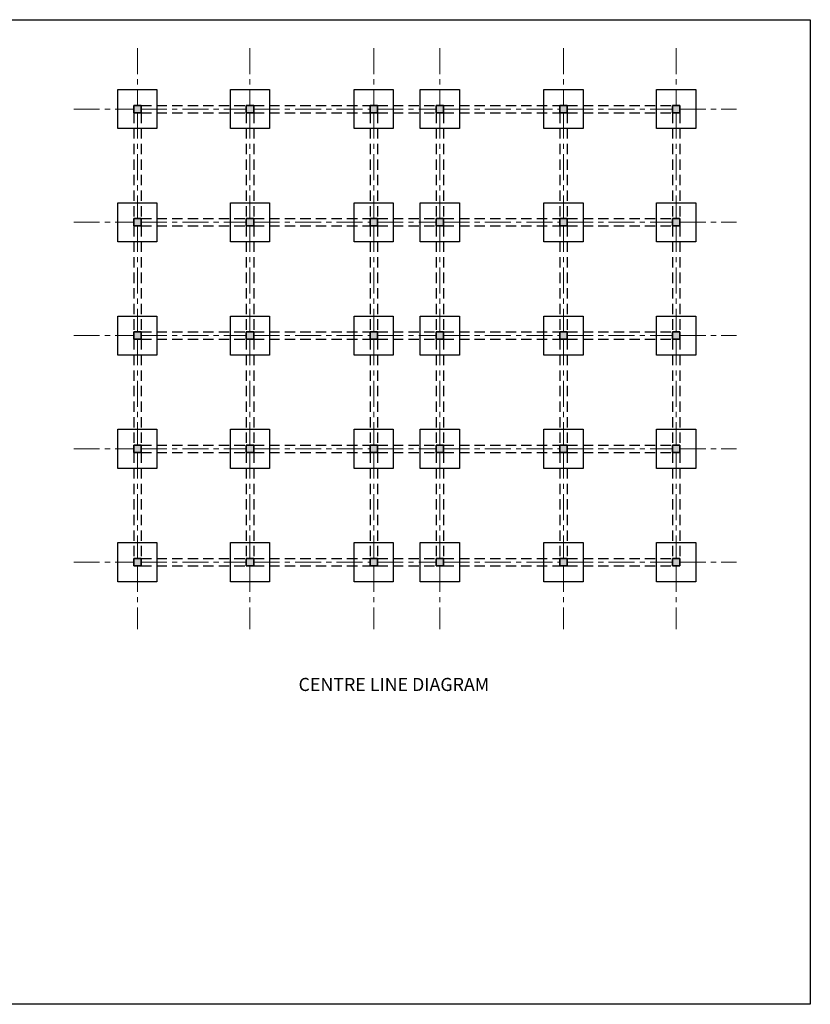
# Model space of a CAD drawing. Units: inches. Extents: x 9239 to 26065, y 6728 to 14611.
# Tile 4 of 12: x 10240 to 11208, y 6728 to 7934. Entities that reach past the tile are written whole.
import ezdxf

# ---------------------------------------------------------------- set-up
doc = ezdxf.new("R2010")
doc.units = ezdxf.units.IN
doc.header["$MEASUREMENT"] = 0
doc.linetypes.add('CENTER', pattern=[50.8, 31.75, -6.35, 6.35, -6.35])
doc.linetypes.add('DASHED', pattern=[19.05, 12.7, -6.35])
for name, color, linetype, lineweight in [('A-ANNO-TEXT', 7, 'Continuous', 18), ('A-FLOR-STRS', 3, 'Continuous', 25), ('A-GRID', 3, 'CENTER', 18), ('S-BEAM', 4, 'DASHED', 25), ('S-COLS', 1, 'Continuous', 35), ('S-FNDN', 6, 'Continuous', 25), ('S-PATT', 252, 'Continuous', 13)]:
    doc.layers.add(name, color=color, linetype=linetype, lineweight=lineweight)
doc.styles.get("Standard").update_dxf_attribs({"font": 'arial.ttf'})

msp = doc.modelspace()

# ---------------------------------------------------------------- hatches: boundary and pattern name
at = {"layer": 'S-PATT'}
h = msp.add_hatch(color=256, dxfattribs=at)
h.dxf.hatch_style = 1
h.paths.add_polyline_path([(10388.37, 7820.07), (10388.37, 7829.07), (10379.37, 7829.07), (10379.37, 7820.07)])
h.paths.add_polyline_path([(10517.37, 7829.07), (10517.37, 7820.07), (10526.37, 7820.07), (10526.37, 7829.07)])
h.paths.add_polyline_path([(10668.87, 7820.07), (10677.87, 7820.07), (10677.87, 7829.07), (10668.87, 7829.07)])
h.paths.add_polyline_path([(10758.87, 7820.07), (10758.87, 7829.07), (10749.87, 7829.07), (10749.87, 7820.07)])
h.paths.add_polyline_path([(10910.37, 7829.07), (10901.37, 7829.07), (10901.37, 7820.07), (10910.37, 7820.07)])
h.paths.add_polyline_path([(11048.37, 7829.07), (11039.37, 7829.07), (11039.37, 7820.07), (11048.37, 7820.07)])
h.paths.add_polyline_path([(10379.37, 7681.32), (10388.37, 7681.32), (10388.37, 7690.32), (10379.37, 7690.32)])
h.paths.add_polyline_path([(10526.37, 7681.32), (10526.37, 7690.32), (10517.37, 7690.32), (10517.37, 7681.32)])
h.paths.add_polyline_path([(10668.87, 7681.32), (10677.87, 7681.32), (10677.87, 7690.32), (10668.87, 7690.32)])
h.paths.add_polyline_path([(10758.87, 7681.32), (10758.87, 7690.32), (10749.87, 7690.32), (10749.87, 7681.32)])
h.paths.add_polyline_path([(10910.37, 7690.32), (10901.37, 7690.32), (10901.37, 7681.32), (10910.37, 7681.32)])
h.paths.add_polyline_path([(11039.37, 7690.32), (11039.37, 7681.32), (11048.37, 7681.32), (11048.37, 7690.32)])
h.paths.add_polyline_path([(10388.37, 7551.57), (10379.37, 7551.57), (10379.37, 7542.57), (10388.37, 7542.57)])
h.paths.add_polyline_path([(10526.37, 7542.57), (10526.37, 7551.57), (10517.37, 7551.57), (10517.37, 7542.57)])
h.paths.add_polyline_path([(10677.87, 7551.57), (10668.87, 7551.57), (10668.87, 7542.57), (10677.87, 7542.57)])
h.paths.add_polyline_path([(10749.87, 7542.57), (10758.87, 7542.57), (10758.87, 7551.57), (10749.87, 7551.57)])
h.paths.add_polyline_path([(10910.37, 7551.57), (10901.37, 7551.57), (10901.37, 7542.57), (10910.37, 7542.57)])
h.paths.add_polyline_path([(11048.37, 7542.57), (11048.37, 7551.57), (11039.37, 7551.57), (11039.37, 7542.57)])
h.paths.add_polyline_path([(10388.37, 7403.82), (10388.37, 7412.82), (10379.37, 7412.82), (10379.37, 7403.82)])
h.paths.add_polyline_path([(10517.37, 7403.82), (10526.37, 7403.82), (10526.37, 7412.82), (10517.37, 7412.82)])
h.paths.add_polyline_path([(10668.87, 7403.82), (10677.87, 7403.82), (10677.87, 7412.82), (10668.87, 7412.82)])
h.paths.add_polyline_path([(10749.87, 7403.82), (10758.87, 7403.82), (10758.87, 7412.82), (10749.87, 7412.82)])
h.paths.add_polyline_path([(10910.37, 7412.82), (10901.37, 7412.82), (10901.37, 7403.82), (10910.37, 7403.82)])
h.paths.add_polyline_path([(11048.37, 7403.82), (11048.37, 7412.82), (11039.37, 7412.82), (11039.37, 7403.82)])
h.paths.add_polyline_path([(11048.37, 7265.07), (11048.37, 7274.07), (11039.37, 7274.07), (11039.37, 7265.07)])
h.paths.add_polyline_path([(10901.37, 7265.07), (10910.37, 7265.07), (10910.37, 7274.07), (10901.37, 7274.07)])
h.paths.add_polyline_path([(10758.87, 7265.07), (10758.87, 7274.07), (10749.87, 7274.07), (10749.87, 7265.07)])
h.paths.add_polyline_path([(10668.87, 7265.07), (10677.87, 7265.07), (10677.87, 7274.07), (10668.87, 7274.07)])
h.paths.add_polyline_path([(10517.37, 7265.07), (10526.37, 7265.07), (10526.37, 7274.07), (10517.37, 7274.07)])
h.paths.add_polyline_path([(10379.37, 7274.07), (10379.37, 7265.07), (10388.37, 7265.07), (10388.37, 7274.07)])

# ---------------------------------------------------------------- linework, layer by layer
at = {"layer": 'A-FLOR-STRS'}
msp.add_lwpolyline([(9238.6, 7933.95), (11208.24, 7933.95), (11208.24, 6728.19), (9238.6, 6728.19)], close=True, dxfattribs=at)
at = {"layer": 'A-GRID'}
for p, q in [((10383.87, 7899.11), (10383.87, 7829.07)), ((10521.87, 7899.11), (10521.87, 7829.07)), ((10673.37, 7899.11), (10673.37, 7829.07)), ((10754.37, 7899.11), (10754.37, 7829.07)), ((10905.87, 7899.11), (10905.87, 7829.07)), ((11043.87, 7899.11), (11043.87, 7829.07)), ((10305.95, 7824.57), (10379.37, 7824.57)), ((10383.87, 7820.07), (10383.87, 7800.57)), ((10383.87, 7820.07), (10383.87, 7690.32)), ((10388.37, 7824.57), (10517.37, 7824.57)), ((10521.87, 7820.07), (10521.87, 7690.32)), ((10526.37, 7824.57), (10668.87, 7824.57)), ((10673.37, 7820.07), (10673.37, 7690.32)), ((10677.87, 7824.57), (10749.87, 7824.57)), ((10754.37, 7820.07), (10754.37, 7690.32)), ((10758.87, 7824.57), (10901.37, 7824.57)), ((10905.87, 7820.07), (10905.87, 7690.32)), ((10910.37, 7824.57), (11039.37, 7824.57)), ((11043.87, 7820.07), (11043.87, 7690.32)), ((11048.37, 7824.57), (11117.64, 7824.57)), ((10305.95, 7685.82), (10379.37, 7685.82)), ((10383.87, 7681.32), (10383.87, 7551.57)), ((10388.37, 7685.82), (10517.37, 7685.82)), ((10521.87, 7681.32), (10521.87, 7551.57)), ((10526.37, 7685.82), (10668.87, 7685.82)), ((10673.37, 7681.32), (10673.37, 7551.57)), ((10677.87, 7685.82), (10749.87, 7685.82)), ((10754.37, 7681.32), (10754.37, 7551.57)), ((10758.87, 7685.82), (10901.37, 7685.82)), ((10905.87, 7681.32), (10905.87, 7551.57)), ((10910.37, 7685.82), (11039.37, 7685.82)), ((11043.87, 7681.32), (11043.87, 7551.57)), ((11048.37, 7685.82), (11117.64, 7685.82)), ((10305.95, 7547.07), (10379.37, 7547.07)), ((10383.87, 7542.57), (10383.87, 7412.82)), ((10388.37, 7547.07), (10517.37, 7547.07)), ((10521.87, 7542.57), (10521.87, 7412.82)), ((10526.37, 7547.07), (10668.87, 7547.07)), ((10673.37, 7542.57), (10673.37, 7412.82)), ((10677.87, 7547.07), (10749.87, 7547.07)), ((10754.37, 7542.57), (10754.37, 7412.82)), ((10758.87, 7547.07), (10901.37, 7547.07)), ((10905.87, 7542.57), (10905.87, 7412.82)), ((10910.37, 7547.07), (11039.37, 7547.07)), ((11043.87, 7542.57), (11043.87, 7412.82)), ((11048.37, 7547.07), (11117.64, 7547.07)), ((10305.95, 7408.32), (10379.37, 7408.32)), ((10383.87, 7403.82), (10383.87, 7274.07)), ((10388.37, 7408.32), (10517.37, 7408.32)), ((10521.87, 7403.82), (10521.87, 7274.07)), ((10526.37, 7408.32), (10668.87, 7408.32)), ((10673.37, 7403.82), (10673.37, 7274.07)), ((10677.87, 7408.32), (10749.87, 7408.32)), ((10754.37, 7403.82), (10754.37, 7274.07)), ((10758.87, 7408.32), (10901.37, 7408.32)), ((10905.87, 7403.82), (10905.87, 7274.07)), ((10910.37, 7408.32), (11039.37, 7408.32)), ((11043.87, 7403.82), (11043.87, 7274.07)), ((11048.37, 7408.32), (11117.64, 7408.32)), ((10305.95, 7269.57), (10379.37, 7269.57)), ((10383.87, 7265.07), (10383.87, 7187.6)), ((10388.37, 7269.57), (10517.37, 7269.57)), ((10521.87, 7265.07), (10521.87, 7187.6)), ((10526.37, 7269.57), (10668.87, 7269.57)), ((10673.37, 7265.07), (10673.37, 7187.6)), ((10677.87, 7269.57), (10749.87, 7269.57)), ((10677.87, 7269.57), (10749.87, 7269.57)), ((10754.37, 7265.07), (10754.37, 7187.6)), ((10758.87, 7269.57), (10901.37, 7269.57)), ((10905.87, 7265.07), (10905.87, 7187.6)), ((10910.37, 7269.57), (11039.37, 7269.57)), ((11043.87, 7265.07), (11043.87, 7187.6)), ((11048.37, 7269.57), (11117.64, 7269.57))]:
    msp.add_line(p, q, dxfattribs=at)
at = {"layer": 'S-BEAM'}
for p, q in [((10388.37, 7829.07), (10517.37, 7829.07)), ((10526.37, 7829.07), (10668.87, 7829.07)), ((10677.87, 7829.07), (10749.87, 7829.07)), ((10758.87, 7829.07), (10901.37, 7829.07)), ((10910.37, 7829.07), (11039.37, 7829.07)), ((10379.37, 7820.07), (10379.37, 7690.32)), ((10388.37, 7820.07), (10388.37, 7690.32)), ((10388.37, 7820.07), (10517.37, 7820.07)), ((10517.37, 7820.07), (10517.37, 7690.32)), ((10526.37, 7820.07), (10526.37, 7690.32)), ((10526.37, 7820.07), (10668.87, 7820.07)), ((10668.87, 7820.07), (10668.87, 7690.32)), ((10677.87, 7820.07), (10677.87, 7690.32)), ((10677.87, 7820.07), (10749.87, 7820.07)), ((10749.87, 7820.07), (10749.87, 7690.32)), ((10758.87, 7820.07), (10758.87, 7690.32)), ((10758.87, 7820.07), (10901.37, 7820.07)), ((10901.37, 7820.07), (10901.37, 7690.32)), ((10910.37, 7820.07), (10910.37, 7690.32)), ((10910.37, 7820.07), (11039.37, 7820.07)), ((11039.37, 7820.07), (11039.37, 7690.32)), ((11048.37, 7820.07), (11048.37, 7690.32)), ((10379.37, 7681.32), (10379.37, 7551.57)), ((10388.37, 7690.32), (10517.37, 7690.32)), ((10388.37, 7681.32), (10388.37, 7551.57)), ((10388.37, 7681.32), (10517.37, 7681.32)), ((10517.37, 7681.32), (10517.37, 7551.57)), ((10526.37, 7690.32), (10668.87, 7690.32)), ((10526.37, 7681.32), (10526.37, 7551.57)), ((10526.37, 7681.32), (10668.87, 7681.32)), ((10668.87, 7681.32), (10668.87, 7551.57)), ((10677.87, 7690.32), (10749.87, 7690.32)), ((10677.87, 7681.32), (10677.87, 7551.57)), ((10677.87, 7681.32), (10749.87, 7681.32)), ((10749.87, 7681.32), (10749.87, 7551.57)), ((10758.87, 7690.32), (10901.37, 7690.32)), ((10758.87, 7681.32), (10758.87, 7551.57)), ((10758.87, 7681.32), (10901.37, 7681.32)), ((10901.37, 7681.32), (10901.37, 7551.57)), ((10910.37, 7690.32), (11039.37, 7690.32)), ((10910.37, 7681.32), (10910.37, 7551.57)), ((10910.37, 7681.32), (11039.37, 7681.32)), ((11039.37, 7681.32), (11039.37, 7551.57)), ((11048.37, 7681.32), (11048.37, 7551.57)), ((10388.37, 7551.57), (10517.37, 7551.57)), ((10526.37, 7551.57), (10668.87, 7551.57)), ((10677.87, 7551.57), (10749.87, 7551.57)), ((10758.87, 7551.57), (10901.37, 7551.57)), ((10910.37, 7551.57), (11039.37, 7551.57)), ((10379.37, 7542.57), (10379.37, 7412.82)), ((10388.37, 7542.57), (10388.37, 7412.82)), ((10388.37, 7542.57), (10517.37, 7542.57)), ((10517.37, 7542.57), (10517.37, 7412.82)), ((10526.37, 7542.57), (10526.37, 7412.82)), ((10526.37, 7542.57), (10668.87, 7542.57)), ((10668.87, 7542.57), (10668.87, 7412.82)), ((10677.87, 7542.57), (10677.87, 7412.82)), ((10677.87, 7542.57), (10749.87, 7542.57)), ((10749.87, 7542.57), (10749.87, 7412.82)), ((10758.87, 7542.57), (10758.87, 7412.82)), ((10758.87, 7542.57), (10901.37, 7542.57)), ((10901.37, 7542.57), (10901.37, 7412.82)), ((10910.37, 7542.57), (10910.37, 7412.82)), ((10910.37, 7542.57), (11039.37, 7542.57)), ((11039.37, 7542.57), (11039.37, 7412.82)), ((11048.37, 7542.57), (11048.37, 7412.82)), ((10379.37, 7403.82), (10379.37, 7274.07)), ((10388.37, 7412.82), (10517.37, 7412.82)), ((10388.37, 7403.82), (10388.37, 7274.07)), ((10388.37, 7403.82), (10517.37, 7403.82)), ((10517.37, 7403.82), (10517.37, 7274.07)), ((10526.37, 7412.82), (10668.87, 7412.82)), ((10526.37, 7403.82), (10526.37, 7274.07)), ((10526.37, 7403.82), (10668.87, 7403.82)), ((10668.87, 7403.82), (10668.87, 7274.07)), ((10677.87, 7412.82), (10749.87, 7412.82)), ((10677.87, 7403.82), (10677.87, 7274.07)), ((10677.87, 7403.82), (10749.87, 7403.82)), ((10749.87, 7403.82), (10749.87, 7274.07)), ((10758.87, 7412.82), (10901.37, 7412.82)), ((10758.87, 7403.82), (10758.87, 7274.07)), ((10758.87, 7403.82), (10901.37, 7403.82)), ((10901.37, 7403.82), (10901.37, 7274.07)), ((10910.37, 7412.82), (11039.37, 7412.82)), ((10910.37, 7403.82), (10910.37, 7274.07)), ((10910.37, 7403.82), (11039.37, 7403.82)), ((11039.37, 7403.82), (11039.37, 7274.07)), ((11048.37, 7403.82), (11048.37, 7274.07)), ((10388.37, 7274.07), (10517.37, 7274.07)), ((10526.37, 7274.07), (10668.87, 7274.07)), ((10677.87, 7274.07), (10749.87, 7274.07)), ((10758.87, 7274.07), (10901.37, 7274.07)), ((10910.37, 7274.07), (11039.37, 7274.07)), ((10388.37, 7265.07), (10517.37, 7265.07)), ((10526.37, 7265.07), (10668.87, 7265.07)), ((10677.87, 7265.07), (10749.87, 7265.07)), ((10758.87, 7265.07), (10901.37, 7265.07)), ((10910.37, 7265.07), (11039.37, 7265.07))]:
    msp.add_line(p, q, dxfattribs=at)
at = {"layer": 'S-COLS'}
for p, q in [((10379.37, 7829.07), (10388.37, 7829.07)), ((10379.37, 7820.07), (10379.37, 7829.07)), ((10388.37, 7829.07), (10388.37, 7820.07)), ((10517.37, 7829.07), (10526.37, 7829.07)), ((10517.37, 7820.07), (10517.37, 7829.07)), ((10526.37, 7829.07), (10526.37, 7820.07)), ((10668.87, 7829.07), (10677.87, 7829.07)), ((10668.87, 7820.07), (10668.87, 7829.07)), ((10677.87, 7829.07), (10677.87, 7820.07)), ((10749.87, 7829.07), (10758.87, 7829.07)), ((10749.87, 7820.07), (10749.87, 7829.07)), ((10758.87, 7829.07), (10758.87, 7820.07)), ((10901.37, 7829.07), (10910.37, 7829.07)), ((10901.37, 7820.07), (10901.37, 7829.07)), ((10910.37, 7829.07), (10910.37, 7820.07)), ((11039.37, 7829.07), (11048.37, 7829.07)), ((11039.37, 7820.07), (11039.37, 7829.07)), ((11048.37, 7829.07), (11048.37, 7820.07)), ((10388.37, 7820.07), (10379.37, 7820.07)), ((10380.87, 7820.07), (10386.87, 7820.07)), ((10526.37, 7820.07), (10517.37, 7820.07)), ((10518.87, 7820.07), (10524.87, 7820.07)), ((10668.87, 7820.07), (10677.87, 7820.07)), ((10677.87, 7820.07), (10668.87, 7820.07)), ((10749.87, 7820.07), (10758.87, 7820.07)), ((10758.87, 7820.07), (10749.87, 7820.07)), ((10910.37, 7820.07), (10901.37, 7820.07)), ((10902.87, 7820.07), (10908.87, 7820.07)), ((11048.37, 7820.07), (11039.37, 7820.07)), ((11040.87, 7820.07), (11046.87, 7820.07)), ((10379.37, 7690.32), (10388.37, 7690.32)), ((10379.37, 7681.32), (10379.37, 7690.32)), ((10388.37, 7681.32), (10379.37, 7681.32)), ((10388.37, 7690.32), (10388.37, 7681.32)), ((10517.37, 7690.32), (10526.37, 7690.32)), ((10517.37, 7681.32), (10517.37, 7690.32)), ((10526.37, 7681.32), (10517.37, 7681.32)), ((10526.37, 7690.32), (10526.37, 7681.32)), ((10668.87, 7690.32), (10677.87, 7690.32)), ((10668.87, 7681.32), (10668.87, 7690.32)), ((10677.87, 7681.32), (10668.87, 7681.32)), ((10677.87, 7690.32), (10677.87, 7681.32)), ((10749.87, 7690.32), (10758.87, 7690.32)), ((10749.87, 7681.32), (10749.87, 7690.32)), ((10758.87, 7681.32), (10749.87, 7681.32)), ((10758.87, 7690.32), (10758.87, 7681.32)), ((10901.37, 7690.32), (10910.37, 7690.32)), ((10901.37, 7681.32), (10901.37, 7690.32)), ((10910.37, 7681.32), (10901.37, 7681.32)), ((10910.37, 7690.32), (10910.37, 7681.32)), ((11039.37, 7690.32), (11048.37, 7690.32)), ((11039.37, 7681.32), (11039.37, 7690.32)), ((11048.37, 7681.32), (11039.37, 7681.32)), ((11048.37, 7690.32), (11048.37, 7681.32)), ((10379.37, 7551.57), (10388.37, 7551.57)), ((10379.37, 7542.57), (10379.37, 7551.57)), ((10388.37, 7551.57), (10388.37, 7542.57)), ((10517.37, 7551.57), (10526.37, 7551.57)), ((10517.37, 7542.57), (10517.37, 7551.57)), ((10526.37, 7551.57), (10526.37, 7542.57)), ((10668.87, 7551.57), (10677.87, 7551.57)), ((10668.87, 7542.57), (10668.87, 7551.57)), ((10677.87, 7551.57), (10677.87, 7542.57)), ((10749.87, 7551.57), (10758.87, 7551.57)), ((10749.87, 7542.57), (10749.87, 7551.57)), ((10758.87, 7551.57), (10758.87, 7542.57)), ((10901.37, 7551.57), (10910.37, 7551.57)), ((10901.37, 7542.57), (10901.37, 7551.57)), ((10910.37, 7551.57), (10910.37, 7542.57)), ((11039.37, 7551.57), (11048.37, 7551.57)), ((11039.37, 7542.57), (11039.37, 7551.57)), ((11048.37, 7551.57), (11048.37, 7542.57)), ((10388.37, 7542.57), (10379.37, 7542.57)), ((10526.37, 7542.57), (10517.37, 7542.57)), ((10677.87, 7542.57), (10668.87, 7542.57)), ((10758.87, 7542.57), (10749.87, 7542.57)), ((10910.37, 7542.57), (10901.37, 7542.57)), ((11048.37, 7542.57), (11039.37, 7542.57)), ((10379.37, 7412.82), (10388.37, 7412.82)), ((10379.37, 7403.82), (10379.37, 7412.82)), ((10388.37, 7403.82), (10379.37, 7403.82)), ((10388.37, 7412.82), (10388.37, 7403.82)), ((10517.37, 7412.82), (10526.37, 7412.82)), ((10517.37, 7403.82), (10517.37, 7412.82)), ((10526.37, 7403.82), (10517.37, 7403.82)), ((10526.37, 7412.82), (10526.37, 7403.82)), ((10668.87, 7412.82), (10677.87, 7412.82)), ((10668.87, 7403.82), (10668.87, 7412.82)), ((10677.87, 7403.82), (10668.87, 7403.82)), ((10677.87, 7412.82), (10677.87, 7403.82)), ((10749.87, 7412.82), (10758.87, 7412.82)), ((10749.87, 7403.82), (10749.87, 7412.82)), ((10758.87, 7403.82), (10749.87, 7403.82)), ((10758.87, 7412.82), (10758.87, 7403.82)), ((10901.37, 7412.82), (10910.37, 7412.82)), ((10901.37, 7403.82), (10901.37, 7412.82)), ((10910.37, 7403.82), (10901.37, 7403.82)), ((10910.37, 7412.82), (10910.37, 7403.82)), ((11039.37, 7412.82), (11048.37, 7412.82)), ((11039.37, 7403.82), (11039.37, 7412.82)), ((11048.37, 7403.82), (11039.37, 7403.82)), ((11048.37, 7412.82), (11048.37, 7403.82)), ((10379.37, 7274.07), (10388.37, 7274.07)), ((10379.37, 7265.07), (10379.37, 7274.07)), ((10388.37, 7274.07), (10388.37, 7265.07)), ((10517.37, 7274.07), (10526.37, 7274.07)), ((10517.37, 7265.07), (10517.37, 7274.07)), ((10526.37, 7274.07), (10526.37, 7265.07)), ((10668.87, 7274.07), (10677.87, 7274.07)), ((10668.87, 7265.07), (10668.87, 7274.07)), ((10677.87, 7274.07), (10677.87, 7265.07)), ((10749.87, 7274.07), (10758.87, 7274.07)), ((10749.87, 7265.07), (10749.87, 7274.07)), ((10758.87, 7274.07), (10758.87, 7265.07)), ((10901.37, 7274.07), (10910.37, 7274.07)), ((10901.37, 7265.07), (10901.37, 7274.07)), ((10910.37, 7274.07), (10910.37, 7265.07)), ((11039.37, 7274.07), (11048.37, 7274.07)), ((11039.37, 7265.07), (11039.37, 7274.07)), ((11048.37, 7274.07), (11048.37, 7265.07)), ((10388.37, 7265.07), (10379.37, 7265.07)), ((10526.37, 7265.07), (10517.37, 7265.07)), ((10677.87, 7265.07), (10668.87, 7265.07)), ((10758.87, 7265.07), (10749.87, 7265.07)), ((10910.37, 7265.07), (10901.37, 7265.07)), ((11048.37, 7265.07), (11039.37, 7265.07))]:
    msp.add_line(p, q, dxfattribs=at)
at = {"layer": 'S-FNDN'}
for p, q in [((10359.87, 7848.57), (10407.87, 7848.57)), ((10359.87, 7800.57), (10359.87, 7848.57)), ((10407.87, 7848.57), (10407.87, 7800.57)), ((10497.87, 7848.57), (10545.87, 7848.57)), ((10497.87, 7800.57), (10497.87, 7848.57)), ((10545.87, 7848.57), (10545.87, 7800.57)), ((10649.37, 7848.57), (10697.37, 7848.57)), ((10649.37, 7800.57), (10649.37, 7848.57)), ((10697.37, 7848.57), (10697.37, 7800.57)), ((10730.37, 7848.57), (10778.37, 7848.57)), ((10730.37, 7800.57), (10730.37, 7848.57)), ((10778.37, 7848.57), (10778.37, 7800.57)), ((10881.87, 7848.57), (10929.87, 7848.57)), ((10881.87, 7800.57), (10881.87, 7848.57)), ((10929.87, 7848.57), (10929.87, 7800.57)), ((11019.87, 7848.57), (11067.87, 7848.57)), ((11019.87, 7800.57), (11019.87, 7848.57)), ((11067.87, 7848.57), (11067.87, 7800.57)), ((10407.87, 7800.57), (10359.87, 7800.57)), ((10545.87, 7800.57), (10497.87, 7800.57)), ((10697.37, 7800.57), (10649.37, 7800.57)), ((10778.37, 7800.57), (10730.37, 7800.57)), ((10929.87, 7800.57), (10881.87, 7800.57)), ((11067.87, 7800.57), (11019.87, 7800.57)), ((10359.87, 7709.82), (10407.87, 7709.82)), ((10359.87, 7661.82), (10359.87, 7709.82)), ((10407.87, 7709.82), (10407.87, 7661.82)), ((10497.87, 7709.82), (10545.87, 7709.82)), ((10497.87, 7661.82), (10497.87, 7709.82)), ((10545.87, 7709.82), (10545.87, 7661.82)), ((10649.37, 7709.82), (10697.37, 7709.82)), ((10649.37, 7661.82), (10649.37, 7709.82)), ((10697.37, 7709.82), (10697.37, 7661.82)), ((10730.37, 7709.82), (10778.37, 7709.82)), ((10730.37, 7661.82), (10730.37, 7709.82)), ((10778.37, 7709.82), (10778.37, 7661.82)), ((10881.87, 7709.82), (10929.87, 7709.82)), ((10881.87, 7661.82), (10881.87, 7709.82)), ((10929.87, 7709.82), (10929.87, 7661.82)), ((11019.87, 7709.82), (11067.87, 7709.82)), ((11019.87, 7661.82), (11019.87, 7709.82)), ((11067.87, 7709.82), (11067.87, 7661.82)), ((10407.87, 7661.82), (10359.87, 7661.82)), ((10545.87, 7661.82), (10497.87, 7661.82)), ((10697.37, 7661.82), (10649.37, 7661.82)), ((10778.37, 7661.82), (10730.37, 7661.82)), ((10929.87, 7661.82), (10881.87, 7661.82)), ((11067.87, 7661.82), (11019.87, 7661.82)), ((10359.87, 7571.07), (10407.87, 7571.07)), ((10359.87, 7523.07), (10359.87, 7571.07)), ((10407.87, 7571.07), (10407.87, 7523.07)), ((10497.87, 7571.07), (10545.87, 7571.07)), ((10497.87, 7523.07), (10497.87, 7571.07)), ((10545.87, 7571.07), (10545.87, 7523.07)), ((10649.37, 7571.07), (10697.37, 7571.07)), ((10649.37, 7523.07), (10649.37, 7571.07)), ((10697.37, 7571.07), (10697.37, 7523.07)), ((10730.37, 7571.07), (10778.37, 7571.07)), ((10730.37, 7523.07), (10730.37, 7571.07)), ((10778.37, 7571.07), (10778.37, 7523.07)), ((10881.87, 7571.07), (10929.87, 7571.07)), ((10881.87, 7523.07), (10881.87, 7571.07)), ((10929.87, 7571.07), (10929.87, 7523.07)), ((11019.87, 7571.07), (11067.87, 7571.07)), ((11019.87, 7523.07), (11019.87, 7571.07)), ((11067.87, 7571.07), (11067.87, 7523.07)), ((10407.87, 7523.07), (10359.87, 7523.07)), ((10545.87, 7523.07), (10497.87, 7523.07)), ((10697.37, 7523.07), (10649.37, 7523.07)), ((10778.37, 7523.07), (10730.37, 7523.07)), ((10929.87, 7523.07), (10881.87, 7523.07)), ((11067.87, 7523.07), (11019.87, 7523.07)), ((10359.87, 7432.32), (10407.87, 7432.32)), ((10359.87, 7384.32), (10359.87, 7432.32)), ((10407.87, 7432.32), (10407.87, 7384.32)), ((10497.87, 7432.32), (10545.87, 7432.32)), ((10497.87, 7384.32), (10497.87, 7432.32)), ((10545.87, 7432.32), (10545.87, 7384.32)), ((10649.37, 7432.32), (10697.37, 7432.32)), ((10649.37, 7384.32), (10649.37, 7432.32)), ((10697.37, 7432.32), (10697.37, 7384.32)), ((10730.37, 7432.32), (10778.37, 7432.32)), ((10730.37, 7384.32), (10730.37, 7432.32)), ((10778.37, 7432.32), (10778.37, 7384.32)), ((10881.87, 7432.32), (10929.87, 7432.32)), ((10881.87, 7384.32), (10881.87, 7432.32)), ((10929.87, 7432.32), (10929.87, 7384.32)), ((11019.87, 7432.32), (11067.87, 7432.32)), ((11019.87, 7384.32), (11019.87, 7432.32)), ((11067.87, 7432.32), (11067.87, 7384.32)), ((10407.87, 7384.32), (10359.87, 7384.32)), ((10545.87, 7384.32), (10497.87, 7384.32)), ((10697.37, 7384.32), (10649.37, 7384.32)), ((10778.37, 7384.32), (10730.37, 7384.32)), ((10929.87, 7384.32), (10881.87, 7384.32)), ((11067.87, 7384.32), (11019.87, 7384.32)), ((10359.87, 7293.57), (10407.87, 7293.57)), ((10359.87, 7245.57), (10359.87, 7293.57)), ((10407.87, 7293.57), (10407.87, 7245.57)), ((10497.87, 7293.57), (10545.87, 7293.57)), ((10497.87, 7245.57), (10497.87, 7293.57)), ((10545.87, 7293.57), (10545.87, 7245.57)), ((10649.37, 7293.57), (10697.37, 7293.57)), ((10649.37, 7245.57), (10649.37, 7293.57)), ((10697.37, 7293.57), (10697.37, 7245.57)), ((10730.37, 7293.57), (10778.37, 7293.57)), ((10730.37, 7245.57), (10730.37, 7293.57)), ((10778.37, 7293.57), (10778.37, 7245.57)), ((10881.87, 7293.57), (10929.87, 7293.57)), ((10881.87, 7245.57), (10881.87, 7293.57)), ((10929.87, 7293.57), (10929.87, 7245.57)), ((11019.87, 7293.57), (11067.87, 7293.57)), ((11019.87, 7245.57), (11019.87, 7293.57)), ((11067.87, 7293.57), (11067.87, 7245.57)), ((10407.87, 7245.57), (10359.87, 7245.57)), ((10545.87, 7245.57), (10497.87, 7245.57)), ((10697.37, 7245.57), (10649.37, 7245.57)), ((10778.37, 7245.57), (10730.37, 7245.57)), ((10929.87, 7245.57), (10881.87, 7245.57)), ((11067.87, 7245.57), (11019.87, 7245.57))]:
    msp.add_line(p, q, dxfattribs=at)

# ---------------------------------------------------------------- texts
at = {"layer": 'A-ANNO-TEXT', "insert": (10581.35, 7127.87), "char_height": 16, "attachment_point": 1}
msp.add_mtext_dynamic_manual_height_columns('CENTRE LINE DIAGRAM', width=738.1388, gutter_width=1, heights=[0], dxfattribs=at)

doc.saveas('drawing.dxf')
